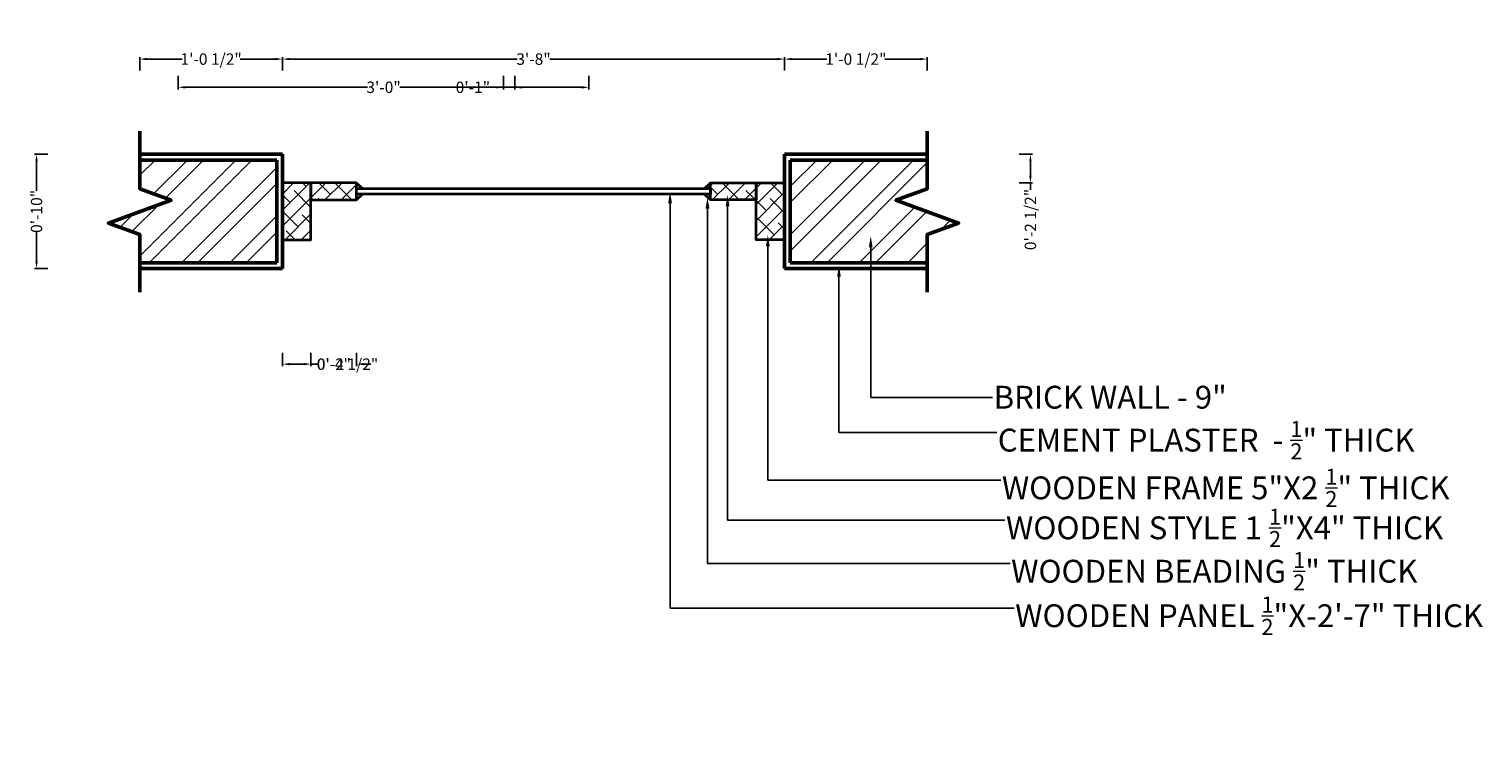
# Model space of a CAD drawing. Units: inches. Extents: x -9 to 130, y -140 to 44.
# Tile 1 of 2: x 3 to 130, y -140 to -78. Entities that reach past the tile are written whole.
import ezdxf
from ezdxf import colors
from ezdxf.entities.mleader import LeaderData, LeaderLine
from ezdxf.math import Vec2, Vec3

# ---------------------------------------------------------------- set-up
doc = ezdxf.new("R2010")
doc.units = ezdxf.units.IN
doc.header["$LTSCALE"] = 3
doc.header["$MEASUREMENT"] = 0
for name, color, linetype, lineweight in [('A-ANNO-DIMS', 2, 'Continuous', 18), ('A-ANNO-TEXT', 3, 'Continuous', 18), ('A-DOOR', 4, 'Continuous', 35), ('A-DOOR-PATT', 9, 'Continuous', 13), ('A-WALL', 7, 'Continuous', 50), ('A-WALL-PATT', 8, 'Continuous', 13)]:
    doc.layers.add(name, color=color, linetype=linetype, lineweight=lineweight)
doc.styles.get("Standard").update_dxf_attribs({"font": 'arial.ttf'})
doc.dimstyles.get("Standard").update_dxf_attribs({"dimtxt": 1, "dimasz": 0.625, "dimexe": 0.18, "dimexo": 0.0625, "dimgap": 0.09, "dimtad": 0, "dimzin": 0, "dimdsep": 46, "dimlunit": 4, "dimtxsty": 'Standard', "dimcen": 0.09, "dimadec": 0, "dimazin": 0, "dimtfac": 1, "dimtofl": 0, "dimtmove": 0, "dimatfit": 3, "dimfxl": 1, "dimfxlon": 1, "dimtolj": 1, "dimtzin": 0, "dimarcsym": 0})

# ---------------------------------------------------------------- blocks, each defined once
blk = doc.blocks.new('DOOR-FRAME-SECT')
at = {"ltscale": 3}
for p, q in [((0.51, 5), (0, 4.5)), ((0.51, 3.5), (0, 4))]:
    blk.add_line(p, q, dxfattribs=at)
for points in [[(0.51, 5), (4.51, 5), (4.51, 3.5), (0.51, 3.5)], [(4.51, 5), (7.01, 5), (7.01, 0), (4.51, 0)]]:
    blk.add_lwpolyline(points, close=True, dxfattribs=at)
blk = doc.blocks.new('*D18')
at = {"layer": 'A-ANNO-DIMS', "color": 0, "lineweight": -2, "ltscale": 3, "transparency": 16777216}
for p, q in [((15.65, -82.24), (15.65, -83.42)), ((51.65, -82.24), (51.65, -83.42)), ((16.27, -83.24), (32.23, -83.24)), ((51.02, -83.24), (35.07, -83.24))]:
    blk.add_line(p, q, dxfattribs=at)
at = {"layer": 'A-ANNO-DIMS', "color": 0, "ltscale": 3, "transparency": 16777216}
for points in [[(16.27, -83.14), (16.27, -83.35), (15.65, -83.24)], [(51.02, -83.14), (51.02, -83.35), (51.65, -83.24)]]:
    blk.add_solid(points, dxfattribs=at)
at = {"layer": 'Defpoints', "color": 0, "ltscale": 3, "transparency": 16777216}
for p in [(15.65, -62.97), (51.65, -62.97), (51.65, -83.24)]:
    blk.add_point(p, dxfattribs=at)
at = {"layer": 'A-ANNO-DIMS', "color": 0, "ltscale": 3, "transparency": 16777216, "insert": (33.65, -83.24), "char_height": 1, "attachment_point": 5}
blk.add_mtext('\\A1;3\'-0"', dxfattribs=at)
blk = doc.blocks.new('*D23')
at = {"layer": 'A-ANNO-DIMS', "color": 0, "lineweight": -2, "ltscale": 3, "transparency": 16777216}
for p, q in [((44.15, -82.24), (44.15, -83.42)), ((45.15, -82.24), (45.15, -83.42)), ((43.52, -83.24), (42.9, -83.24)), ((45.77, -83.24), (46.4, -83.24))]:
    blk.add_line(p, q, dxfattribs=at)
at = {"layer": 'A-ANNO-DIMS', "color": 0, "ltscale": 3, "transparency": 16777216}
for points in [[(43.52, -83.14), (43.52, -83.35), (44.15, -83.24)], [(45.77, -83.14), (45.77, -83.35), (45.15, -83.24)]]:
    blk.add_solid(points, dxfattribs=at)
at = {"layer": 'Defpoints', "color": 0, "ltscale": 3, "transparency": 16777216}
for p in [(44.15, -54.47), (45.15, -55.47), (44.15, -83.24)]:
    blk.add_point(p, dxfattribs=at)
at = {"layer": 'A-ANNO-DIMS', "color": 0, "ltscale": 3, "transparency": 16777216, "insert": (41.48, -83.24), "char_height": 1, "attachment_point": 5}
blk.add_mtext('\\A1;0\'-1"', dxfattribs=at)
blk = doc.blocks.new('*D27')
at = {"layer": 'A-ANNO-DIMS', "color": 0, "lineweight": -2, "ltscale": 3, "transparency": 16777216}
for p, q in [((12.29, -81.77), (12.29, -80.59)), ((12.92, -80.77), (16, -80.77)), ((24.17, -80.77), (21.08, -80.77)), ((24.79, -81.77), (24.79, -80.59))]:
    blk.add_line(p, q, dxfattribs=at)
at = {"layer": 'A-ANNO-DIMS', "color": 0, "ltscale": 3, "transparency": 16777216}
for points in [[(12.92, -80.66), (12.92, -80.87), (12.29, -80.77)], [(24.17, -80.66), (24.17, -80.87), (24.79, -80.77)]]:
    blk.add_solid(points, dxfattribs=at)
at = {"layer": 'Defpoints', "color": 0, "ltscale": 3, "transparency": 16777216}
for p in [(24.79, -80.77), (12.29, -89.11), (24.79, -89.11)]:
    blk.add_point(p, dxfattribs=at)
at = {"layer": 'A-ANNO-DIMS', "color": 0, "ltscale": 3, "transparency": 16777216, "insert": (18.54, -80.77), "char_height": 1, "attachment_point": 5}
blk.add_mtext('\\A1;1\'-0 1/2"', dxfattribs=at)
blk = doc.blocks.new('*D28')
at = {"layer": 'A-ANNO-DIMS', "color": 0, "lineweight": -2, "ltscale": 3, "transparency": 16777216}
for p, q in [((24.79, -81.77), (24.79, -80.59)), ((25.42, -80.77), (45.37, -80.77)), ((68.17, -80.77), (48.21, -80.77)), ((68.79, -81.77), (68.79, -80.59))]:
    blk.add_line(p, q, dxfattribs=at)
at = {"layer": 'A-ANNO-DIMS', "color": 0, "ltscale": 3, "transparency": 16777216}
for points in [[(25.42, -80.66), (25.42, -80.87), (24.79, -80.77)], [(68.17, -80.66), (68.17, -80.87), (68.79, -80.77)]]:
    blk.add_solid(points, dxfattribs=at)
at = {"layer": 'Defpoints', "color": 0, "ltscale": 3, "transparency": 16777216}
for p in [(68.79, -80.77), (24.79, -89.11), (68.79, -89.11)]:
    blk.add_point(p, dxfattribs=at)
at = {"layer": 'A-ANNO-DIMS', "color": 0, "ltscale": 3, "transparency": 16777216, "insert": (46.79, -80.77), "char_height": 1, "attachment_point": 5}
blk.add_mtext('\\A1;3\'-8"', dxfattribs=at)
blk = doc.blocks.new('*D29')
at = {"layer": 'A-ANNO-DIMS', "color": 0, "lineweight": -2, "ltscale": 3, "transparency": 16777216}
for p, q in [((68.79, -81.77), (68.79, -80.59)), ((69.42, -80.77), (72.5, -80.77)), ((80.67, -80.77), (77.58, -80.77)), ((81.29, -81.77), (81.29, -80.59))]:
    blk.add_line(p, q, dxfattribs=at)
at = {"layer": 'A-ANNO-DIMS', "color": 0, "ltscale": 3, "transparency": 16777216}
for points in [[(69.42, -80.66), (69.42, -80.87), (68.79, -80.77)], [(80.67, -80.66), (80.67, -80.87), (81.29, -80.77)]]:
    blk.add_solid(points, dxfattribs=at)
at = {"layer": 'Defpoints', "color": 0, "ltscale": 3, "transparency": 16777216}
for p in [(81.29, -80.77), (68.79, -89.11), (81.29, -89.11)]:
    blk.add_point(p, dxfattribs=at)
at = {"layer": 'A-ANNO-DIMS', "color": 0, "ltscale": 3, "transparency": 16777216, "insert": (75.04, -80.77), "char_height": 1, "attachment_point": 5}
blk.add_mtext('\\A1;1\'-0 1/2"', dxfattribs=at)
blk = doc.blocks.new('*D30')
at = {"layer": 'A-ANNO-DIMS', "color": 0, "lineweight": -2, "ltscale": 3, "transparency": 16777216}
for p, q in [((4.24, -89.11), (3.06, -89.11)), ((3.24, -89.73), (3.24, -92.3)), ((3.24, -98.48), (3.24, -95.92)), ((4.24, -99.11), (3.06, -99.11))]:
    blk.add_line(p, q, dxfattribs=at)
at = {"layer": 'A-ANNO-DIMS', "color": 0, "ltscale": 3, "transparency": 16777216}
for points in [[(3.14, -89.73), (3.35, -89.73), (3.24, -89.11)], [(3.14, -98.48), (3.35, -98.48), (3.24, -99.11)]]:
    blk.add_solid(points, dxfattribs=at)
at = {"layer": 'Defpoints', "color": 0, "ltscale": 3, "transparency": 16777216}
for p in [(12.29, -89.11), (3.24, -99.11), (12.29, -99.11)]:
    blk.add_point(p, dxfattribs=at)
at = {"layer": 'A-ANNO-DIMS', "color": 0, "ltscale": 3, "transparency": 16777216, "insert": (3.24, -94.11), "char_height": 1, "attachment_point": 5, "rotation": 90}
blk.add_mtext('\\A1;0\'-10"', dxfattribs=at)
blk = doc.blocks.new('*D31')
at = {"layer": 'A-ANNO-DIMS', "color": 0, "lineweight": -2, "ltscale": 3, "transparency": 16777216}
for p, q in [((24.79, -106.49), (24.79, -107.67)), ((27.29, -106.49), (27.29, -107.67)), ((25.42, -107.49), (26.67, -107.49)), ((27.29, -107.49), (27.92, -107.49))]:
    blk.add_line(p, q, dxfattribs=at)
at = {"layer": 'A-ANNO-DIMS', "color": 0, "ltscale": 3, "transparency": 16777216}
for points in [[(25.42, -107.38), (25.42, -107.59), (24.79, -107.49)], [(26.67, -107.38), (26.67, -107.59), (27.29, -107.49)]]:
    blk.add_solid(points, dxfattribs=at)
at = {"layer": 'Defpoints', "color": 0, "ltscale": 3, "transparency": 16777216}
for p in [(24.79, -96.61), (27.29, -96.61), (27.29, -107.49)]:
    blk.add_point(p, dxfattribs=at)
at = {"layer": 'A-ANNO-DIMS', "color": 0, "ltscale": 3, "transparency": 16777216, "insert": (30.5, -107.49), "char_height": 1, "attachment_point": 5}
blk.add_mtext('\\A1;0\'-2 1/2"', dxfattribs=at)
blk = doc.blocks.new('*D32')
at = {"layer": 'A-ANNO-DIMS', "color": 0, "lineweight": -2, "ltscale": 3, "transparency": 16777216}
for p, q in [((27.29, -106.49), (27.29, -107.67)), ((31.29, -106.49), (31.29, -107.67)), ((26.67, -107.49), (26.04, -107.49)), ((31.92, -107.49), (32.54, -107.49))]:
    blk.add_line(p, q, dxfattribs=at)
at = {"layer": 'A-ANNO-DIMS', "color": 0, "ltscale": 3, "transparency": 16777216}
for points in [[(26.67, -107.38), (26.67, -107.59), (27.29, -107.49)], [(31.92, -107.38), (31.92, -107.59), (31.29, -107.49)]]:
    blk.add_solid(points, dxfattribs=at)
at = {"layer": 'Defpoints', "color": 0, "ltscale": 3, "transparency": 16777216}
for p in [(27.29, -93.11), (31.29, -93.11), (31.29, -107.49)]:
    blk.add_point(p, dxfattribs=at)
at = {"layer": 'A-ANNO-DIMS', "color": 0, "ltscale": 3, "transparency": 16777216, "insert": (29.29, -107.49), "char_height": 1, "attachment_point": 5}
blk.add_mtext('\\A1;0\'-4"', dxfattribs=at)
blk = doc.blocks.new('*D33')
at = {"layer": 'A-ANNO-DIMS', "color": 0, "lineweight": -2, "ltscale": 3, "transparency": 16777216}
for p, q in [((89.34, -89.11), (90.52, -89.11)), ((90.34, -89.73), (90.34, -90.98)), ((89.34, -91.61), (90.52, -91.61)), ((90.34, -91.61), (90.34, -92.23))]:
    blk.add_line(p, q, dxfattribs=at)
at = {"layer": 'A-ANNO-DIMS', "color": 0, "ltscale": 3, "transparency": 16777216}
for points in [[(90.23, -89.73), (90.44, -89.73), (90.34, -89.11)], [(90.23, -90.98), (90.44, -90.98), (90.34, -91.61)]]:
    blk.add_solid(points, dxfattribs=at)
at = {"layer": 'Defpoints', "color": 0, "ltscale": 3, "transparency": 16777216}
for p in [(68.79, -89.11), (66.29, -91.61), (90.34, -91.61)]:
    blk.add_point(p, dxfattribs=at)
at = {"layer": 'A-ANNO-DIMS', "color": 0, "ltscale": 3, "transparency": 16777216, "insert": (90.34, -94.82), "char_height": 1, "attachment_point": 5, "rotation": 90}
blk.add_mtext('\\A1;0\'-2 1/2"', dxfattribs=at)

msp = doc.modelspace()

# ---------------------------------------------------------------- hatches: boundary and pattern name
at = {"layer": 'A-DOOR-PATT', "ltscale": 3}
h = msp.add_hatch(dxfattribs=at)
h.set_pattern_fill('ANSI38', color=256, scale=8)
h.paths.add_polyline_path([(68.791, -91.608), (66.291, -91.608), (66.291, -96.608), (68.791, -96.608)])
h.paths.add_polyline_path([(66.291, -91.608), (62.291, -91.608), (62.291, -93.108), (66.291, -93.108)])
h.paths.add_polyline_path([(62.291, -91.608), (61.783, -92.108), (62.291, -92.108)])
h.paths.add_polyline_path([(62.291, -92.608), (61.783, -92.608), (62.291, -93.108)])
h.paths.add_polyline_path([(27.291, -91.608), (24.791, -91.608), (24.791, -96.608), (27.291, -96.608)])
h.paths.add_polyline_path([(31.291, -91.608), (27.291, -91.608), (27.291, -93.108), (31.291, -93.108)])
h = msp.add_hatch(color=256, dxfattribs=at)
h.dxf.hatch_style = 1
h.paths.add_polyline_path([(31.798, -92.608), (31.291, -92.608), (31.291, -93.108)])
h.paths.add_polyline_path([(31.291, -91.608), (31.291, -92.108), (31.798, -92.108)])
h.paths.add_polyline_path([(62.291, -91.608), (61.783, -92.108), (62.291, -92.108)])
h.paths.add_polyline_path([(62.291, -92.608), (61.783, -92.608), (62.291, -93.108)])
at = {"layer": 'A-WALL-PATT', "ltscale": 3}
h = msp.add_hatch(dxfattribs=at)
h.set_pattern_fill('ANSI32', color=256, scale=8)
h.paths.add_polyline_path([(81.291, -96.128), (84.038, -95.128), (78.543, -93.128), (81.291, -92.128), (81.291, -89.608), (69.291, -89.608), (69.291, -98.608), (81.291, -98.608)])
h.paths.add_polyline_path([(24.291, -89.608), (12.291, -89.608), (12.291, -92.128), (15.038, -93.128), (9.543, -95.128), (12.291, -96.128), (12.291, -98.608), (24.291, -98.608)])

# ---------------------------------------------------------------- linework, layer by layer
at = {"layer": 'A-DOOR', "ltscale": 3}
msp.add_lwpolyline([(31.291, -92.108), (62.291, -92.108), (62.291, -92.608), (31.291, -92.608)], close=True, dxfattribs=at)
at = {"layer": 'A-WALL', "ltscale": 3}
for p, q in [((12.291, -89.108), (24.791, -89.108)), ((24.791, -89.108), (24.791, -99.108)), ((81.291, -89.108), (68.791, -89.108)), ((68.791, -89.108), (68.791, -99.108)), ((12.291, -89.608), (24.291, -89.608)), ((24.291, -89.608), (24.291, -98.608)), ((81.291, -89.608), (69.291, -89.608)), ((69.291, -89.608), (69.291, -98.608)), ((24.291, -98.608), (12.291, -98.608)), ((24.791, -99.108), (12.291, -99.108)), ((68.791, -99.108), (81.291, -99.108)), ((69.291, -98.608), (81.291, -98.608))]:
    msp.add_line(p, q, dxfattribs=at)
for points in [[(12.291, -87.069), (12.291, -92.128), (15.038, -93.128), (9.543, -95.128), (12.291, -96.128), (12.291, -101.186)], [(81.291, -87.069), (81.291, -92.128), (78.543, -93.128), (84.038, -95.128), (81.291, -96.128), (81.291, -101.186)]]:
    msp.add_lwpolyline(points, dxfattribs=at)

# ---------------------------------------------------------------- block references
at = {"layer": 'A-DOOR', "extrusion": (0, 0, -1), "zscale": -1}
msp.add_blockref('DOOR-FRAME-SECT', (-31.799, -96.608), dxfattribs=at)
at = {"layer": 'A-DOOR'}
msp.add_blockref('DOOR-FRAME-SECT', (61.783, -96.608), dxfattribs=at)

# ---------------------------------------------------------------- dimensions: what is measured, and where the dimension line sits
at = {"layer": 'A-ANNO-DIMS', "ltscale": 3}
for base, p1, p2, picture, middle in [((44.148, -83.244), (45.148, -55.474), (44.148, -54.474), '*D23', (41.478, -83.244)), ((51.648, -83.244), (15.648, -62.974), (51.648, -62.974), '*D18', (33.648, -83.244)), ((24.791, -80.769), (12.291, -89.108), (24.791, -89.108), '*D27', (18.541, -80.769)), ((68.791, -80.769), (24.791, -89.108), (68.791, -89.108), '*D28', (46.791, -80.769)), ((81.291, -80.769), (68.791, -89.108), (81.291, -89.108), '*D29', (75.041, -80.769)), ((31.291, -107.486), (27.291, -93.108), (31.291, -93.108), '*D32', (29.291, -107.486)), ((27.291, -107.486), (24.791, -96.608), (27.291, -96.608), '*D31', (30.5, -107.486))]:
    dim = msp.add_linear_dim(base=base, p1=p1, p2=p2, dimstyle='Standard', override={"dimdec": 1, "dimlfac": 1, "dimrnd": 0, "dimzin": 1, "dimdsep": 46, "dimlunit": 4, "dimfrac": 2}, dxfattribs=at)
    dim.commit()
    dim.dimension.update_dxf_attribs({"geometry": picture, "text_midpoint": middle})
for base, p1, p2, picture, middle in [((3.243, -99.108), (12.291, -89.108), (12.291, -99.108), '*D30', (3.243, -94.108)), ((90.338, -91.608), (68.791, -89.108), (66.291, -91.608), '*D33', (90.338, -94.817))]:
    dim = msp.add_linear_dim(base=base, p1=p1, p2=p2, angle=90, dimstyle='Standard', override={"dimdec": 1, "dimlfac": 1, "dimrnd": 0, "dimzin": 1, "dimdsep": 46, "dimlunit": 4, "dimfrac": 2}, dxfattribs=at)
    dim.commit()
    dim.dimension.update_dxf_attribs({"geometry": picture, "text_midpoint": middle})

# ---------------------------------------------------------------- leaders
at = {"layer": 'A-ANNO-TEXT', "ltscale": 3}
ml = msp.add_multileader_mtext('Standard', dxfattribs=at)
ml.set_content('\\A1;WOODEN PANEL {\\H0.7x;\\S1/2;}"X-2\'-7" THICK', color=256)
ml.set_leader_properties()
ml.build(insert=Vec2(0, 0))
ml.multileader.update_dxf_attribs({"dogleg_length": 0.36, "arrow_head_size": 1})
ctx = ml.context
ctx.base_point, ctx.char_height, ctx.arrow_head_size, ctx.landing_gap_size, ctx.plane_origin = Vec3(88.915, -128.861), 2, 1, 0.09, Vec3(58.756, -92.399)
notes = []
notes.append((ctx, [(0, (1, 1, 0), (88.555, -128.861), (1, 0), 0.36, [(0, [(58.756, -92.399), (58.756, -128.861)], 0, [])])]))
ctx.mtext.insert, ctx.mtext.flow_direction = Vec3(89.005, -127.843), 5
ml = msp.add_multileader_mtext('Standard', dxfattribs=at)
ml.set_content('\\A1;WOODEN BEADING {\\H0.7x;\\S1/2;}" THICK', color=256)
ml.set_leader_properties()
ml.build(insert=Vec2(0, 0))
ml.multileader.update_dxf_attribs({"dogleg_length": 0.36, "arrow_head_size": 1})
ctx = ml.context
ctx.base_point, ctx.char_height, ctx.arrow_head_size, ctx.landing_gap_size, ctx.plane_origin = Vec3(88.555, -124.964), 2, 1, 0.09, Vec3(62.037, -92.858)
notes.append((ctx, [(0, (1, 1, 0), (88.195, -124.964), (1, 0), 0.36, [(0, [(62.037, -92.858), (62.037, -124.964)], 0, [])])]))
ctx.mtext.insert, ctx.mtext.flow_direction = Vec3(88.645, -123.947), 5
ml = msp.add_multileader_mtext('Standard', dxfattribs=at)
ml.set_content('\\A1;WOODEN STYLE 1 {\\H0.7x;\\S1/2;}"X4" THICK', color=256)
ml.set_leader_properties()
ml.build(insert=Vec2(0, 0))
ml.multileader.update_dxf_attribs({"dogleg_length": 0.36, "arrow_head_size": 1})
ctx = ml.context
ctx.base_point, ctx.char_height, ctx.arrow_head_size, ctx.landing_gap_size, ctx.plane_origin = Vec3(88.105, -121.165), 2, 1, 0.09, Vec3(63.8, -92.653)
notes.append((ctx, [(0, (1, 1, 0), (87.745, -121.165), (1, 0), 0.36, [(0, [(63.8, -92.653), (63.8, -121.165)], 0, [])])]))
ctx.mtext.insert, ctx.mtext.flow_direction = Vec3(88.195, -120.148), 5
ml = msp.add_multileader_mtext('Standard', dxfattribs=at)
ml.set_content('\\A1;WOODEN FRAME 5"X2 {\\H0.7x;\\S1/2;}" THICK', color=256)
ml.set_leader_properties()
ml.build(insert=Vec2(0, 0))
ml.multileader.update_dxf_attribs({"dogleg_length": 0.36, "arrow_head_size": 1})
ctx = ml.context
ctx.base_point, ctx.char_height, ctx.arrow_head_size, ctx.landing_gap_size, ctx.plane_origin = Vec3(87.745, -117.662), 2, 1, 0.09, Vec3(67.327, -96.168)
notes.append((ctx, [(0, (1, 1, 0), (87.385, -117.662), (1, 0), 0.36, [(0, [(67.327, -96.168), (67.327, -117.662)], 0, [])])]))
ctx.mtext.insert, ctx.mtext.flow_direction = Vec3(87.835, -116.645), 5
ml = msp.add_multileader_mtext('Standard', dxfattribs=at)
ml.set_content('BRICK WALL - 9"', color=256)
ml.set_leader_properties()
ml.build(insert=Vec2(0, 0))
ml.multileader.update_dxf_attribs({"dogleg_length": 0.36, "arrow_head_size": 1})
ctx = ml.context
ctx.base_point, ctx.char_height, ctx.arrow_head_size, ctx.landing_gap_size, ctx.plane_origin = Vec3(87.025, -110.402), 2, 1, 0.09, Vec3(76.341, -96.258)
notes.append((ctx, [(0, (1, 1, 0), (86.665, -110.402), (1, 0), 0.36, [(0, [(76.341, -96.258), (76.341, -110.402)], 0, [])])]))
ctx.mtext.insert, ctx.mtext.flow_direction = Vec3(87.115, -109.385), 5
ml = msp.add_multileader_mtext('Standard', dxfattribs=at)
ml.set_content('\\A1;CEMENT PLASTER  - {\\H0.7x;\\S1/2;}" THICK', color=256)
ml.set_leader_properties()
ml.build(insert=Vec2(0, 0))
ml.multileader.update_dxf_attribs({"dogleg_length": 0.36, "arrow_head_size": 1})
ctx = ml.context
ctx.base_point, ctx.char_height, ctx.arrow_head_size, ctx.landing_gap_size, ctx.plane_origin = Vec3(87.385, -113.481), 2, 1, 0.09, Vec3(73.561, -98.839)
notes.append((ctx, [(0, (1, 1, 0), (87.025, -113.481), (1, 0), 0.36, [(0, [(73.561, -98.839), (73.561, -113.481)], 0, [])])]))
ctx.mtext.insert, ctx.mtext.flow_direction = Vec3(87.475, -112.464), 5
for ctx, leaders in notes:
    for number, flags, end, landing, length, lines in leaders:
        leader = LeaderData()
        leader.index, (leader.has_last_leader_line, leader.has_dogleg_vector, leader.attachment_direction) = number, flags
        leader.last_leader_point, leader.dogleg_vector, leader.dogleg_length = Vec3(end), Vec3(landing), length
        for number, points, colour, breaks in lines:
            line = LeaderLine()
            line.index, line.vertices, line.color, line.breaks = number, Vec3.list(points), colors.encode_raw_color(colour), breaks
            leader.lines.append(line)
        ctx.leaders.append(leader)

doc.saveas('drawing.dxf')
